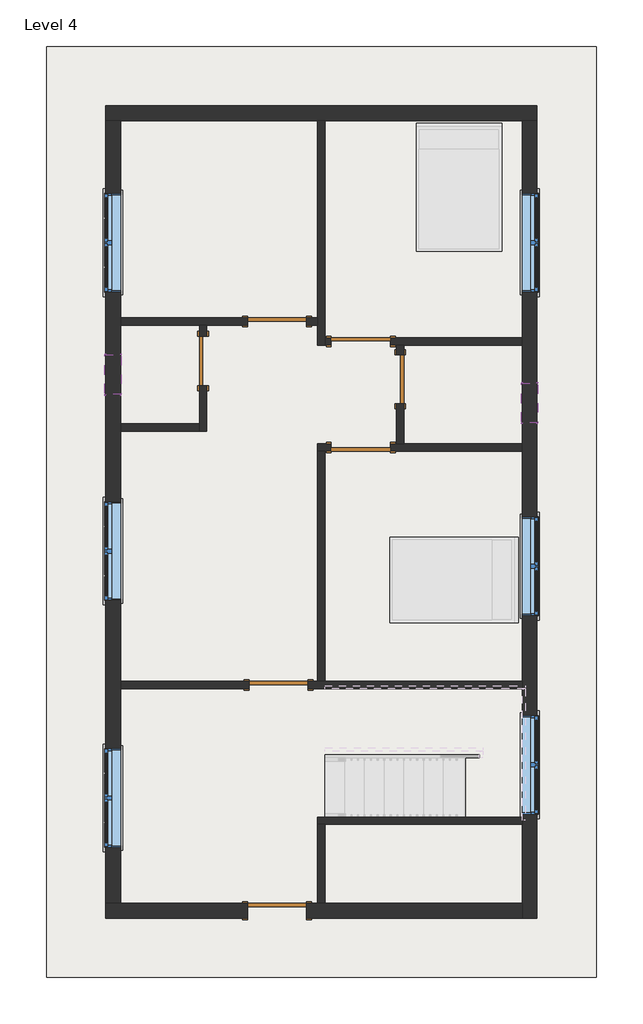
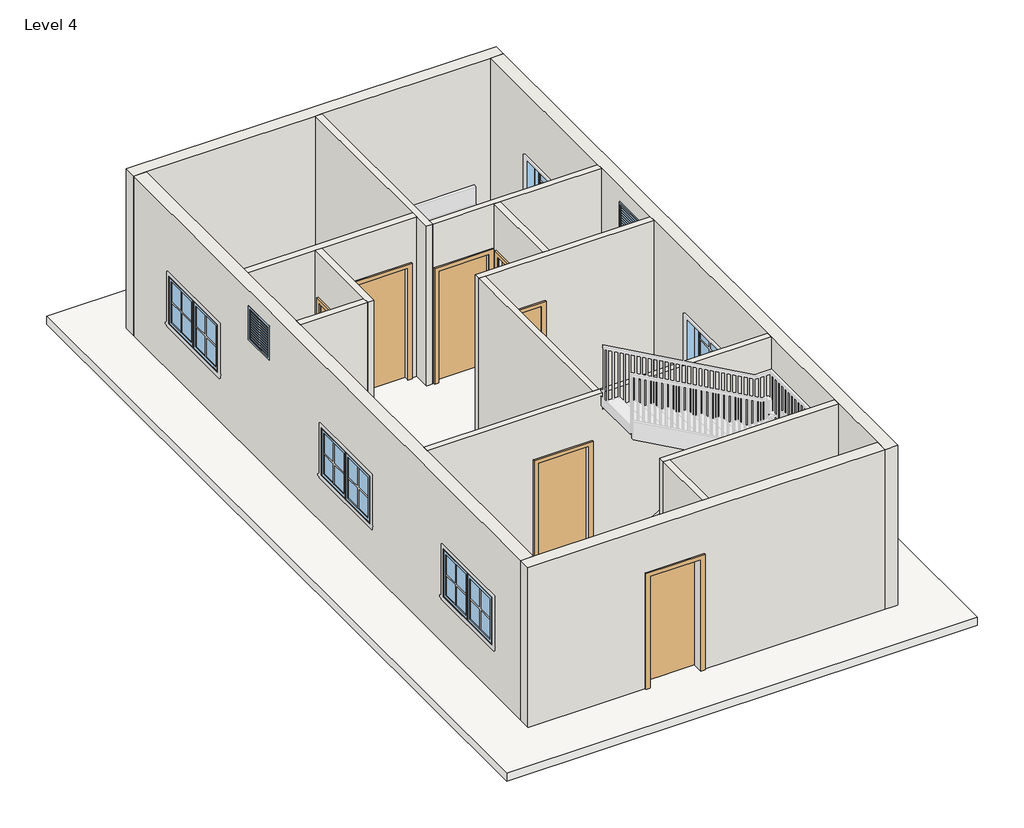
# One storey, part 1 of 3: 15 walls, 8 windows, 7 doors, 1 roof.
"""IFC4 building model written with IfcOpenShell, lengths in millimetres."""

from ifc_helpers import new_model, si_unit, frame, origin, place, context, project, spatial, polyline, outline, extrude, faceted_brep, transform, mapped, element, save
from components import door_78caadf7, door_214872d5, single_flush_door_3_e5f9f3c4, single_flush_door_3_305aa2a5, single_flush_door_3_0ca8825f, window_casement_double_win_5_c1d95f0f, window_f2d8fef0

model = new_model("IFC4")

# Units and contexts
model_context = context("Model", 3, world=origin())
ifc_project = project(units=[si_unit("LENGTHUNIT", "METRE", prefix="MILLI")], contexts=[model_context])

# Site, building, storey
site = spatial("IfcSite", under=ifc_project)
building = spatial("IfcBuilding", under=site)
storey = spatial("IfcBuildingStorey", under=building, Name="Level 4", Elevation=9448.8)

# Doors
placement = place(None, origin())
door_shape = door_78caadf7(model_context)
element("IfcDoor", 1, ObjectType="Single-Flush : 2'6\"", at=placement, inside=storey, context=model_context, shape_type="MappedRepresentation", body=[
    mapped(door_shape, transform((-35.92188, 1946.24131, 9448.8), x_axis=(0.0, 1.0, 0.0), y_axis=(-1.0, 0.0, 0.0), z_axis=(0.0, 0.0, 1.0))),
])
door_2_shape = door_214872d5(model_context)
element("IfcDoor", 2, ObjectType="Single-Flush : 2'6\"", at=placement, inside=storey, context=model_context, shape_type="MappedRepresentation", body=[
    mapped(door_2_shape, transform((-3083.92188, 2225.64131, 9448.8), x_axis=(0.0, 1.0, 0.0), y_axis=(-1.0, 0.0, 0.0), z_axis=(0.0, 0.0, 1.0))),
])
single_flush_door_3_shape = single_flush_door_3_e5f9f3c4(model_context)
element("IfcDoor", 3, ObjectType="Single-Flush : DOOR 3'", at=placement, inside=storey, context=model_context, shape_type="MappedRepresentation", body=[
    mapped(single_flush_door_3_shape, transform((-1940.92188, 2835.24131, 9448.8), x_axis=(1.0, 0.0, 0.0), y_axis=(0.0, 1.0, 0.0), z_axis=(0.0, 0.0, 1.0))),
])
element("IfcDoor", 4, ObjectType="Single-Flush : DOOR 3'", at=placement, inside=storey, context=model_context, shape_type="MappedRepresentation", body=[
    mapped(single_flush_door_3_shape, transform((-645.52188, 892.14131, 9448.8), x_axis=(-1.0, 0.0, 0.0), y_axis=(0.0, -1.0, 0.0), z_axis=(0.0, 0.0, 1.0))),
])
element("IfcDoor", 5, ObjectType="Single-Flush : DOOR 3'", at=placement, inside=storey, context=model_context, shape_type="MappedRepresentation", body=[
    mapped(single_flush_door_3_shape, transform((-1915.52188, -2778.15869, 9448.8), x_axis=(1.0, 0.0, 0.0), y_axis=(0.0, 1.0, 0.0), z_axis=(0.0, 0.0, 1.0))),
])
single_flush_door_3_2_shape = single_flush_door_3_305aa2a5(model_context)
element("IfcDoor", 6, ObjectType="Single-Flush : DOOR 3'", at=placement, inside=storey, context=model_context, shape_type="MappedRepresentation", body=[
    mapped(single_flush_door_3_2_shape, transform((-645.52188, 2530.44131, 9448.8), x_axis=(-1.0, 0.0, 0.0), y_axis=(0.0, -1.0, 0.0), z_axis=(0.0, 0.0, 1.0))),
])
single_flush_door_3_3_shape = single_flush_door_3_0ca8825f(model_context)
element("IfcDoor", 7, ObjectType="Single-Flush : DOOR 3'", at=placement, inside=storey, context=model_context, shape_type="MappedRepresentation", body=[
    mapped(single_flush_door_3_3_shape, transform((-1940.92188, -6264.30869, 9448.8), x_axis=(1.0, 0.0, 0.0), y_axis=(0.0, 1.0, 0.0), z_axis=(0.0, 0.0, 1.0))),
])

# Roof
element("IfcRoof", 8, ObjectType="ROOF 6\"", at=placement, inside=storey, context=model_context, shape_type="SweptSolid", body=[
    extrude(outline(polyline([(-5503.27188, 7083.39131), (2993.02812, 7083.39131), (2993.02812, -7293.00869), (-5503.27188, -7293.00869), (-5503.27188, 7083.39131)])), frame((0.0, 0.0, 9296.4), z_axis=(0.0, 0.0, 1.0), x_axis=(1.0, 0.0, 0.0)), (0.0, 0.0, 1.0), 152.4),
])

# Walls
element("IfcWall", 9, ObjectType="WALL 4.5'", at=placement, inside=storey, context=model_context, shape_type="Brep", body=[
    faceted_brep([(-1312.27188, 5940.39131, 9448.8), (-1312.27188, 2892.39131, 9448.8), (-1312.27188, 2778.09131, 9448.8), (-1312.27188, 2473.29131, 9448.8), (-1312.27188, 2473.29131, 12496.8), (-1312.27188, 2778.09131, 12496.8), (-1312.27188, 2892.39131, 12496.8), (-1312.27188, 5940.39131, 12496.8), (-1197.97188, 5940.39131, 9448.8), (-1197.97188, 5940.39131, 12496.8), (-1197.97188, 2587.59131, 12496.8), (-1197.97188, 2473.29131, 12496.8), (-1197.97188, 2473.29131, 9448.8), (-1197.97188, 2587.59131, 9448.8)], [[[0, 1, 2, 3, 4, 5, 6, 7]], [[8, 9, 10, 11, 12, 13]], [[3, 2, 1, 0, 8, 13, 12]], [[0, 7, 9, 8]], [[4, 3, 12, 11]], [[7, 6, 5, 4, 11, 10, 9]]]),
])
element("IfcWall", 10, ObjectType="WALL 4.5'", at=placement, inside=storey, context=model_context, shape_type="Brep", body=[
    faceted_brep([(-1197.97188, 2473.29131, 9448.8), (-1102.72188, 2473.29131, 9448.8), (-1102.72188, 2473.29131, 11582.4), (-188.32188, 2473.29131, 11582.4), (-188.32188, 2473.29131, 9448.8), (-93.07188, 2473.29131, 9448.8), (21.22812, 2473.29131, 9448.8), (1850.02812, 2473.29131, 9448.8), (1850.02812, 2473.29131, 12496.8), (21.22812, 2473.29131, 12496.8), (-93.07188, 2473.29131, 12496.8), (-1197.97188, 2473.29131, 12496.8), (-1102.72188, 2587.59131, 11582.4), (-1102.72188, 2587.59131, 9448.8), (-1197.97188, 2587.59131, 9448.8), (-1197.97188, 2587.59131, 12496.8), (1850.02812, 2587.59131, 12496.8), (1850.02812, 2587.59131, 9448.8), (-188.32188, 2587.59131, 9448.8), (-188.32188, 2587.59131, 11582.4)], [[[0, 1, 2, 3, 4, 5, 6, 7, 8, 9, 10, 11]], [[12, 13, 14, 15, 16, 17, 18, 19]], [[18, 17, 7, 6, 5, 4]], [[14, 13, 1, 0]], [[0, 11, 15, 14]], [[8, 7, 17, 16]], [[2, 1, 13, 12]], [[3, 2, 12, 19]], [[4, 3, 19, 18]], [[11, 10, 9, 8, 16, 15]]]),
])
element("IfcWall", 11, ObjectType="WALL 4.5'", at=placement, inside=storey, context=model_context, shape_type="Brep", body=[
    faceted_brep([(-1312.27188, 2892.39131, 9448.8), (-1483.72188, 2892.39131, 9448.8), (-1483.72188, 2892.39131, 11582.4), (-2398.12188, 2892.39131, 11582.4), (-2398.12188, 2892.39131, 9448.8), (-4360.27188, 2892.39131, 9448.8), (-4360.27188, 2892.39131, 12496.8), (-1312.27188, 2892.39131, 12496.8), (-1483.72188, 2778.09131, 11582.4), (-1483.72188, 2778.09131, 9448.8), (-1312.27188, 2778.09131, 9448.8), (-1312.27188, 2778.09131, 12496.8), (-3026.77188, 2778.09131, 12496.8), (-3141.07188, 2778.09131, 12496.8), (-4360.27188, 2778.09131, 12496.8), (-4360.27188, 2778.09131, 9448.8), (-3141.07188, 2778.09131, 9448.8), (-3026.77188, 2778.09131, 9448.8), (-2398.12188, 2778.09131, 9448.8), (-2398.12188, 2778.09131, 11582.4)], [[[0, 1, 2, 3, 4, 5, 6, 7]], [[8, 9, 10, 11, 12, 13, 14, 15, 16, 17, 18, 19]], [[10, 9, 1, 0]], [[18, 17, 16, 15, 5, 4]], [[6, 5, 15, 14]], [[0, 7, 11, 10]], [[2, 1, 9, 8]], [[3, 2, 8, 19]], [[4, 3, 19, 18]], [[7, 6, 14, 13, 12, 11]]]),
])
element("IfcWall", 12, ObjectType="WALL 4.5'", at=placement, inside=storey, context=model_context, shape_type="Brep", body=[
    faceted_brep([(-3141.07188, 2778.09131, 9448.8), (-3141.07188, 2606.64131, 9448.8), (-3141.07188, 2606.64131, 11582.4), (-3141.07188, 1844.64131, 11582.4), (-3141.07188, 1844.64131, 9448.8), (-3141.07188, 1254.09131, 9448.8), (-3141.07188, 1139.79131, 9448.8), (-3141.07188, 1139.79131, 12496.8), (-3141.07188, 1254.09131, 12496.8), (-3141.07188, 2778.09131, 12496.8), (-3026.77188, 2606.64131, 11582.4), (-3026.77188, 2606.64131, 9448.8), (-3026.77188, 2778.09131, 9448.8), (-3026.77188, 2778.09131, 12496.8), (-3026.77188, 1139.79131, 12496.8), (-3026.77188, 1139.79131, 9448.8), (-3026.77188, 1844.64131, 9448.8), (-3026.77188, 1844.64131, 11582.4)], [[[0, 1, 2, 3, 4, 5, 6, 7, 8, 9]], [[10, 11, 12, 13, 14, 15, 16, 17]], [[16, 15, 6, 5, 4]], [[12, 11, 1, 0]], [[0, 9, 13, 12]], [[7, 6, 15, 14]], [[2, 1, 11, 10]], [[3, 2, 10, 17]], [[4, 3, 17, 16]], [[9, 8, 7, 14, 13]]]),
])
element("IfcWall", 13, ObjectType="WALL 4.5'", at=placement, inside=storey, context=model_context, shape_type="SweptSolid", body=[
    extrude(outline(polyline([(-4360.27188, 1254.09131), (-3141.07188, 1254.09131), (-3141.07188, 1139.79131), (-4360.27188, 1139.79131), (-4360.27188, 1254.09131)])), frame((0.0, 0.0, 9448.8), z_axis=(0.0, 0.0, 1.0), x_axis=(1.0, 0.0, 0.0)), (0.0, 0.0, 1.0), 3048.0),
])
element("IfcWall", 14, ObjectType="WALL 4.5'", at=placement, inside=storey, context=model_context, shape_type="SweptSolid", body=[
    extrude(outline(polyline([(2473.29131, 9448.8), (2327.24131, 9448.8), (2327.24131, 11582.4), (1565.24131, 11582.4), (1565.24131, 9448.8), (949.29131, 9448.8), (949.29131, 12496.8), (2473.29131, 12496.8), (2473.29131, 9448.8)])), frame((-93.07188, 0.0, 0.0), z_axis=(1.0, 0.0, 0.0), x_axis=(0.0, 1.0, 0.0)), (0.0, 0.0, 1.0), 114.3),
])
element("IfcWall", 15, ObjectType="WALL 4.5'", at=placement, inside=storey, context=model_context, shape_type="Brep", body=[
    faceted_brep([(-1102.72188, 949.29131, 11582.4), (-1102.72188, 949.29131, 9448.8), (-1312.27188, 949.29131, 9448.8), (-1312.27188, 949.29131, 12496.8), (-93.07188, 949.29131, 12496.8), (21.22812, 949.29131, 12496.8), (1850.02812, 949.29131, 12496.8), (1850.02812, 949.29131, 9448.8), (21.22812, 949.29131, 9448.8), (-93.07188, 949.29131, 9448.8), (-188.32188, 949.29131, 9448.8), (-188.32188, 949.29131, 11582.4), (-1312.27188, 834.99131, 9448.8), (-1197.97188, 834.99131, 9448.8), (-1102.72188, 834.99131, 9448.8), (-1102.72188, 834.99131, 11582.4), (-188.32188, 834.99131, 11582.4), (-188.32188, 834.99131, 9448.8), (1850.02812, 834.99131, 9448.8), (1850.02812, 834.99131, 12496.8), (-1197.97188, 834.99131, 12496.8), (-1312.27188, 834.99131, 12496.8)], [[[0, 1, 2, 3, 4, 5, 6, 7, 8, 9, 10, 11]], [[12, 13, 14, 15, 16, 17, 18, 19, 20, 21]], [[2, 1, 14, 13, 12]], [[10, 9, 8, 7, 18, 17]], [[7, 6, 19, 18]], [[3, 2, 12, 21]], [[15, 14, 1, 0]], [[16, 15, 0, 11]], [[17, 16, 11, 10]], [[6, 5, 4, 3, 21, 20, 19]]]),
])
element("IfcWall", 16, ObjectType="WALL 4.5'", at=placement, inside=storey, context=model_context, shape_type="SweptSolid", body=[
    extrude(outline(polyline([(-1312.27188, -2721.00869), (-1312.27188, 834.99131), (-1197.97188, 834.99131), (-1197.97188, -2721.00869), (-1312.27188, -2721.00869)])), frame((0.0, 0.0, 9448.8), z_axis=(0.0, 0.0, 1.0), x_axis=(1.0, 0.0, 0.0)), (0.0, 0.0, 1.0), 3048.0),
])
element("IfcWall", 17, ObjectType="WALL 4.5'", at=placement, inside=storey, context=model_context, shape_type="Brep", body=[
    faceted_brep([(1850.02812, -2721.00869, 9448.8), (-1197.97188, -2721.00869, 9448.8), (-1312.27188, -2721.00869, 9448.8), (-1458.32188, -2721.00869, 9448.8), (-1458.32188, -2721.00869, 11582.4), (-2372.72188, -2721.00869, 11582.4), (-2372.72188, -2721.00869, 9448.8), (-4360.27188, -2721.00869, 9448.8), (-4360.27188, -2721.00869, 12496.8), (-1312.27188, -2721.00869, 12496.8), (-1197.97188, -2721.00869, 12496.8), (1850.02812, -2721.00869, 12496.8), (-1458.32188, -2835.30869, 11582.4), (-1458.32188, -2835.30869, 9448.8), (1850.02812, -2835.30869, 9448.8), (1850.02812, -2835.30869, 12496.8), (-4360.27188, -2835.30869, 12496.8), (-4360.27188, -2835.30869, 9448.8), (-2372.72188, -2835.30869, 9448.8), (-2372.72188, -2835.30869, 11582.4)], [[[0, 1, 2, 3, 4, 5, 6, 7, 8, 9, 10, 11]], [[12, 13, 14, 15, 16, 17, 18, 19]], [[18, 17, 7, 6]], [[14, 13, 3, 2, 1, 0]], [[0, 11, 15, 14]], [[8, 7, 17, 16]], [[4, 3, 13, 12]], [[5, 4, 12, 19]], [[6, 5, 19, 18]], [[11, 10, 9, 8, 16, 15]]]),
])
element("IfcWall", 18, ObjectType="WALL 4.5'", at=placement, inside=storey, context=model_context, shape_type="Brep", body=[
    faceted_brep([(1850.02812, -4816.50869, 9448.8), (-1312.27188, -4816.50869, 9448.8), (-1312.27188, -4816.50869, 12496.8), (1850.02812, -4816.50869, 12496.8), (1850.02812, -4930.80869, 9448.8), (1850.02812, -4930.80869, 12496.8), (-1197.97188, -4930.80869, 12496.8), (-1312.27188, -4930.80869, 12496.8), (-1312.27188, -4930.80869, 9448.8), (-1197.97188, -4930.80869, 9448.8)], [[[0, 1, 2, 3]], [[4, 5, 6, 7, 8, 9]], [[1, 0, 4, 9, 8]], [[0, 3, 5, 4]], [[2, 1, 8, 7]], [[3, 2, 7, 6, 5]]]),
])
element("IfcWall", 19, ObjectType="WALL 4.5'", at=placement, inside=storey, context=model_context, shape_type="SweptSolid", body=[
    extrude(outline(polyline([(-1312.27188, -6150.00869), (-1312.27188, -4930.80869), (-1197.97188, -4930.80869), (-1197.97188, -6150.00869), (-1312.27188, -6150.00869)])), frame((0.0, 0.0, 9448.8), z_axis=(0.0, 0.0, 1.0), x_axis=(1.0, 0.0, 0.0)), (0.0, 0.0, 1.0), 3048.0),
])
element("IfcWall", 20, ObjectType="WALL 9\"", at=placement, inside=storey, context=model_context, shape_type="Brep", body=[
    faceted_brep([(-4588.87188, 5940.39131, 9448.8), (-4360.27188, 5940.39131, 9448.8), (-1312.27188, 5940.39131, 9448.8), (-1197.97188, 5940.39131, 9448.8), (1850.02812, 5940.39131, 9448.8), (2078.62812, 5940.39131, 9448.8), (2078.62812, 5940.39131, 12496.8), (1850.02812, 5940.39131, 12496.8), (-1197.97188, 5940.39131, 12496.8), (-1312.27188, 5940.39131, 12496.8), (-4360.27188, 5940.39131, 12496.8), (-4588.87188, 5940.39131, 12496.8), (-4588.87188, 6168.99131, 9448.8), (-4588.87188, 6168.99131, 12496.8), (2078.62812, 6168.99131, 12496.8), (2078.62812, 6168.99131, 9448.8)], [[[0, 1, 2, 3, 4, 5, 6, 7, 8, 9, 10, 11]], [[12, 13, 14, 15]], [[5, 4, 3, 2, 1, 0, 12, 15]], [[6, 5, 15, 14]], [[0, 11, 13, 12]], [[11, 10, 9, 8, 7, 6, 14, 13]]]),
])
element("IfcWall", 21, ObjectType="WALL 9\"", at=placement, inside=storey, context=model_context, shape_type="Brep", body=[
    faceted_brep([(1850.02812, 5940.39131, 9448.8), (1850.02812, 2587.59131, 9448.8), (1850.02812, 2473.29131, 9448.8), (1850.02812, 949.29131, 9448.8), (1850.02812, 834.99131, 9448.8), (1850.02812, -2721.00869, 9448.8), (1850.02812, -2835.30869, 9448.8), (1850.02812, -4816.50869, 9448.8), (1850.02812, -4930.80869, 9448.8), (1850.02812, -6150.00869, 9448.8), (1850.02812, -6378.60869, 9448.8), (1850.02812, -6378.60869, 12496.8), (1850.02812, -6150.00869, 12496.8), (1850.02812, -4930.80869, 12496.8), (1850.02812, -4816.50869, 12496.8), (1850.02812, -2835.30869, 12496.8), (1850.02812, -2721.00869, 12496.8), (1850.02812, 834.99131, 12496.8), (1850.02812, 949.29131, 12496.8), (1850.02812, 2473.29131, 12496.8), (1850.02812, 2587.59131, 12496.8), (1850.02812, 5940.39131, 12496.8), (1850.02812, -4772.05869, 11277.6), (1850.02812, -4772.05869, 10363.2), (1850.02812, -3248.05869, 10363.2), (1850.02812, -3248.05869, 11277.6), (1850.02812, 3292.44131, 11277.6), (1850.02812, 3292.44131, 10363.2), (1850.02812, 4816.44131, 10363.2), (1850.02812, 4816.44131, 11277.6), (1850.02812, -1705.00869, 11277.6), (1850.02812, -1705.00869, 10363.2), (1850.02812, -181.00869, 10363.2), (1850.02812, -181.00869, 11277.6), (1850.02812, 1273.14131, 12192.0), (1850.02812, 1273.14131, 11582.4), (1850.02812, 1882.74131, 11582.4), (1850.02812, 1882.74131, 12192.0), (2078.62812, 5940.39131, 9448.8), (2078.62812, 5940.39131, 12496.8), (2078.62812, -6378.60869, 12496.8), (2078.62812, -6378.60869, 9448.8), (2078.62812, -4772.05869, 11277.6), (2078.62812, -3248.05869, 11277.6), (2078.62812, -3248.05869, 10363.2), (2078.62812, -4772.05869, 10363.2), (2078.62812, 3292.44131, 11277.6), (2078.62812, 4816.44131, 11277.6), (2078.62812, 4816.44131, 10363.2), (2078.62812, 3292.44131, 10363.2), (2078.62812, -1705.00869, 11277.6), (2078.62812, -181.00869, 11277.6), (2078.62812, -181.00869, 10363.2), (2078.62812, -1705.00869, 10363.2), (2078.62812, 1273.14131, 12192.0), (2078.62812, 1882.74131, 12192.0), (2078.62812, 1882.74131, 11582.4), (2078.62812, 1273.14131, 11582.4)], [[[0, 1, 2, 3, 4, 5, 6, 7, 8, 9, 10, 11, 12, 13, 14, 15, 16, 17, 18, 19, 20, 21], [22, 23, 24, 25], [26, 27, 28, 29], [30, 31, 32, 33], [34, 35, 36, 37]], [[38, 39, 40, 41], [42, 43, 44, 45], [46, 47, 48, 49], [50, 51, 52, 53], [54, 55, 56, 57]], [[10, 9, 8, 7, 6, 5, 4, 3, 2, 1, 0, 38, 41]], [[0, 21, 39, 38]], [[11, 10, 41, 40]], [[23, 22, 42, 45]], [[24, 23, 45, 44]], [[25, 24, 44, 43]], [[22, 25, 43, 42]], [[27, 26, 46, 49]], [[28, 27, 49, 48]], [[29, 28, 48, 47]], [[26, 29, 47, 46]], [[31, 30, 50, 53]], [[32, 31, 53, 52]], [[33, 32, 52, 51]], [[30, 33, 51, 50]], [[35, 34, 54, 57]], [[36, 35, 57, 56]], [[37, 36, 56, 55]], [[34, 37, 55, 54]], [[21, 20, 19, 18, 17, 16, 15, 14, 13, 12, 11, 40, 39]]]),
])
element("IfcWall", 22, ObjectType="WALL 9\"", at=placement, inside=storey, context=model_context, shape_type="Brep", body=[
    faceted_brep([(1850.02812, -6150.00869, 9448.8), (-1197.97188, -6150.00869, 9448.8), (-1312.27188, -6150.00869, 9448.8), (-1483.72188, -6150.00869, 9448.8), (-1483.72188, -6150.00869, 11582.4), (-2398.12188, -6150.00869, 11582.4), (-2398.12188, -6150.00869, 9448.8), (-4360.27188, -6150.00869, 9448.8), (-4588.87188, -6150.00869, 9448.8), (-4588.87188, -6150.00869, 12496.8), (-4360.27188, -6150.00869, 12496.8), (-1312.27188, -6150.00869, 12496.8), (-1197.97188, -6150.00869, 12496.8), (1850.02812, -6150.00869, 12496.8), (-1483.72188, -6378.60869, 11582.4), (-1483.72188, -6378.60869, 9448.8), (1850.02812, -6378.60869, 9448.8), (1850.02812, -6378.60869, 12496.8), (-4588.87188, -6378.60869, 12496.8), (-4588.87188, -6378.60869, 9448.8), (-2398.12188, -6378.60869, 9448.8), (-2398.12188, -6378.60869, 11582.4)], [[[0, 1, 2, 3, 4, 5, 6, 7, 8, 9, 10, 11, 12, 13]], [[14, 15, 16, 17, 18, 19, 20, 21]], [[20, 19, 8, 7, 6]], [[16, 15, 3, 2, 1, 0]], [[0, 13, 17, 16]], [[9, 8, 19, 18]], [[4, 3, 15, 14]], [[5, 4, 14, 21]], [[6, 5, 21, 20]], [[13, 12, 11, 10, 9, 18, 17]]]),
])
element("IfcWall", 23, ObjectType="WALL 9\"", at=placement, inside=storey, context=model_context, shape_type="Brep", body=[
    faceted_brep([(-4360.27188, -6150.00869, 9448.8), (-4360.27188, -2835.30869, 9448.8), (-4360.27188, -2721.00869, 9448.8), (-4360.27188, 1139.79131, 9448.8), (-4360.27188, 1254.09131, 9448.8), (-4360.27188, 2778.09131, 9448.8), (-4360.27188, 2892.39131, 9448.8), (-4360.27188, 5940.39131, 9448.8), (-4360.27188, 5940.39131, 12496.8), (-4360.27188, 2892.39131, 12496.8), (-4360.27188, 2778.09131, 12496.8), (-4360.27188, 1254.09131, 12496.8), (-4360.27188, 1139.79131, 12496.8), (-4360.27188, -2721.00869, 12496.8), (-4360.27188, -2835.30869, 12496.8), (-4360.27188, -6150.00869, 12496.8), (-4360.27188, 4816.44131, 11277.6), (-4360.27188, 4816.44131, 10363.2), (-4360.27188, 3292.44131, 10363.2), (-4360.27188, 3292.44131, 11277.6), (-4360.27188, 53.94131, 11277.6), (-4360.27188, 53.94131, 10363.2), (-4360.27188, -1470.05869, 10363.2), (-4360.27188, -1470.05869, 11277.6), (-4360.27188, -3759.23369, 11277.6), (-4360.27188, -3759.23369, 10363.2), (-4360.27188, -5283.23369, 10363.2), (-4360.27188, -5283.23369, 11277.6), (-4360.27188, 1711.29131, 12192.0), (-4360.27188, 2320.89131, 12192.0), (-4360.27188, 2320.89131, 11582.4), (-4360.27188, 1711.29131, 11582.4), (-4588.87188, -6150.00869, 9448.8), (-4588.87188, -6150.00869, 12496.8), (-4588.87188, 5940.39131, 12496.8), (-4588.87188, 5940.39131, 9448.8), (-4588.87188, 4816.44131, 11277.6), (-4588.87188, 3292.44131, 11277.6), (-4588.87188, 3292.44131, 10363.2), (-4588.87188, 4816.44131, 10363.2), (-4588.87188, 53.94131, 11277.6), (-4588.87188, -1470.05869, 11277.6), (-4588.87188, -1470.05869, 10363.2), (-4588.87188, 53.94131, 10363.2), (-4588.87188, -3759.23369, 11277.6), (-4588.87188, -5283.23369, 11277.6), (-4588.87188, -5283.23369, 10363.2), (-4588.87188, -3759.23369, 10363.2), (-4588.87188, 1711.29131, 12192.0), (-4588.87188, 1711.29131, 11582.4), (-4588.87188, 2320.89131, 11582.4), (-4588.87188, 2320.89131, 12192.0)], [[[0, 1, 2, 3, 4, 5, 6, 7, 8, 9, 10, 11, 12, 13, 14, 15], [16, 17, 18, 19], [20, 21, 22, 23], [24, 25, 26, 27], [28, 29, 30, 31]], [[32, 33, 34, 35], [36, 37, 38, 39], [40, 41, 42, 43], [44, 45, 46, 47], [48, 49, 50, 51]], [[7, 6, 5, 4, 3, 2, 1, 0, 32, 35]], [[8, 7, 35, 34]], [[0, 15, 33, 32]], [[17, 16, 36, 39]], [[18, 17, 39, 38]], [[19, 18, 38, 37]], [[16, 19, 37, 36]], [[21, 20, 40, 43]], [[22, 21, 43, 42]], [[23, 22, 42, 41]], [[20, 23, 41, 40]], [[25, 24, 44, 47]], [[26, 25, 47, 46]], [[27, 26, 46, 45]], [[24, 27, 45, 44]], [[49, 48, 28, 31]], [[50, 49, 31, 30]], [[51, 50, 30, 29]], [[48, 51, 29, 28]], [[15, 14, 13, 12, 11, 10, 9, 8, 34, 33]]]),
])

# Windows
window_casement_double_win_5_shape = window_casement_double_win_5_c1d95f0f(model_context)
element("IfcWindow", 24, ObjectType="Window-Casement-Double : WIN 5'", at=placement, inside=storey, context=model_context, shape_type="MappedRepresentation", body=[
    mapped(window_casement_double_win_5_shape, transform((-4474.57188, 4054.44131, 9448.8), x_axis=(0.0, 1.0, 0.0), y_axis=(-1.0, 0.0, 0.0), z_axis=(0.0, 0.0, 1.0))),
])
element("IfcWindow", 25, ObjectType="Window-Casement-Double : WIN 5'", at=placement, inside=storey, context=model_context, shape_type="MappedRepresentation", body=[
    mapped(window_casement_double_win_5_shape, transform((-4474.57188, -708.05869, 9448.8), x_axis=(0.0, 1.0, 0.0), y_axis=(-1.0, 0.0, 0.0), z_axis=(0.0, 0.0, 1.0))),
])
element("IfcWindow", 26, ObjectType="Window-Casement-Double : WIN 5'", at=placement, inside=storey, context=model_context, shape_type="MappedRepresentation", body=[
    mapped(window_casement_double_win_5_shape, transform((-4474.57188, -4521.23369, 9448.8), x_axis=(0.0, 1.0, 0.0), y_axis=(-1.0, 0.0, 0.0), z_axis=(0.0, 0.0, 1.0))),
])
element("IfcWindow", 27, ObjectType="Window-Casement-Double : WIN 5'", at=placement, inside=storey, context=model_context, shape_type="MappedRepresentation", body=[
    mapped(window_casement_double_win_5_shape, transform((1964.32812, -4010.05869, 9448.8), x_axis=(0.0, -1.0, 0.0), y_axis=(1.0, 0.0, 0.0), z_axis=(0.0, 0.0, 1.0))),
])
element("IfcWindow", 28, ObjectType="Window-Casement-Double : WIN 5'", at=placement, inside=storey, context=model_context, shape_type="MappedRepresentation", body=[
    mapped(window_casement_double_win_5_shape, transform((1964.32812, 4054.44131, 9448.8), x_axis=(0.0, -1.0, 0.0), y_axis=(1.0, 0.0, 0.0), z_axis=(0.0, 0.0, 1.0))),
])
element("IfcWindow", 29, ObjectType="Window-Casement-Double : WIN 5'", at=placement, inside=storey, context=model_context, shape_type="MappedRepresentation", body=[
    mapped(window_casement_double_win_5_shape, transform((1964.32812, -943.00869, 9448.8), x_axis=(0.0, -1.0, 0.0), y_axis=(1.0, 0.0, 0.0), z_axis=(0.0, 0.0, 1.0))),
])
window_shape = window_f2d8fef0(model_context)
element("IfcWindow", 30, ObjectType="Window-Louvers : 24\" x 24\"", at=placement, inside=storey, context=model_context, shape_type="MappedRepresentation", body=[
    mapped(window_shape, transform((1957.97812, 1577.94131, 10668.0), x_axis=(0.0, 1.0, 0.0), y_axis=(-1.0, 0.0, 0.0), z_axis=(0.0, 0.0, 1.0))),
])
element("IfcWindow", 31, ObjectType="Window-Louvers : 24\" x 24\"", at=placement, inside=storey, context=model_context, shape_type="MappedRepresentation", body=[
    mapped(window_shape, transform((-4480.92188, 2016.09131, 10668.0), x_axis=(0.0, 1.0, 0.0), y_axis=(-1.0, 0.0, 0.0), z_axis=(0.0, 0.0, 1.0))),
])

save(model, "model.ifc")

# Revit data of these elements
# Type "Single-Flush : 2'6\""
#   Type Mark = "9"
#   Construction Type Id = "MDOOR"
#   Assembly Code = "C1020"
#   Analytic Construction = "Metal"
#   Thickness = 0' - 2"
#   Heat Transfer Coefficient (U) = 0.651978 BTU/(h·ft²·°F)
#   Height = 7' - 0"
#   Trim Projection Ext = 0' - 1"
#   Trim Projection Int = 0' - 1"
#   Trim Width = 0' - 3"
#   Width = 2' - 6"
#   Define Thermal Properties by = 1
#   Door Material = Door - Panel
#   Frame Material = Door - Frame
#   Visual Light Transmittance = 0
#   Solar Heat Gain Coefficient = 0
#   Function = (empty or 0)
#   Wall Closure = (empty or 0)
# Type "Single-Flush : DOOR 3'"
#   Type Mark = "8"
#   Construction Type Id = "MDOOR"
#   Assembly Code = "C1020"
#   Analytic Construction = "Metal"
#   Thickness = 0' - 2"
#   Heat Transfer Coefficient (U) = 0.651978 BTU/(h·ft²·°F)
#   Height = 7' - 0"
#   Trim Projection Ext = 0' - 1"
#   Trim Projection Int = 0' - 1"
#   Trim Width = 0' - 3"
#   Width = 3' - 0"
#   Define Thermal Properties by = 1
#   Door Material = Door - Panel
#   Frame Material = Door - Frame
#   Visual Light Transmittance = 0
#   Solar Heat Gain Coefficient = 0
#   Function = (empty or 0)
#   Wall Closure = (empty or 0)
# Type "ROOF 6\""
#   Assembly Code = "B1020"
#   Layers, outside or top first: 0' - 6" no material (function 1)
# Type "WALL 4.5'"
#   Assembly Code = "B2010"
#   Layers, outside or top first: 0' - 4 1/2" no material (function 1)
# Type "WALL 9\""
#   Assembly Code = "B2010"
#   Layers, outside or top first: 0' - 9" no material (function 1)
# Type "Window-Casement-Double : WIN 5'"
#   Type Mark = "18"
#   Fire Rating = "0.5h"
#   Assembly Code = "B2020100"
#   Analytic Construction = "Double glazing - domestic"
#   Frame Extension [instance default] = 0' - 0 1/4"
#   Window Inset [instance default] = 0' - 0"
#   Wall Thickness [instance default] = 0' - 6"
#   Interior Wall Closure [instance default] = 0' - 2 1/4"
#   Half Width = 2' - 6"
#   Visual Light Transmittance = 0.81
#   Thermal Resistance (R) = 1.8146 (h·ft²·°F)/BTU
#   Solar Heat Gain Coefficient = 0.76
#   Rough Width = 5' - 0 1/2"
#   Rough Height = 3' - 0 1/2"
#   Height = 3' - 0"
#   Heat Transfer Coefficient (U) = 0.5511 BTU/(h·ft²·°F)
#   Exterior Wall Closure [instance default] = 0' - 1 1/4"
#   Extension Jamb [instance default] = 0' - 2 1/4"
#   Default Sill Height = 3' - 0"
#   Width = 5' - 0"
#   Muntin Visibility = yes
#   Interior Trim Visibility [instance default] = yes
#   Exterior Trim Visibility [instance default] = yes
#   Extension Jamb Visibility [instance default] = yes
#   Interior Trim Material = Wood - Stained
#   Muntin Pattern = Muntin Pattern_2x2 : Muntin Pattern_2x2
#   Interior Trim = Trim-Window-Interior-Flat : Picture Frame
#   Interior Frame Material = Wood - Stained
#   Glass Panel Material = Glass
#   Exterior Trim Material = Clad - White
#   Exterior Trim = Trim-Window-Exterior-Flat : with Sill
#   Exterior Frame Material = Clad - White
#   Wall Closure = (empty or 0)
# Type "Window-Louvers : 24\" x 24\""
#   Type Mark = "19"
#   Construction Type Id = "GSP4R"
#   Assembly Code = "B20"
#   Analytic Construction = "1/8 in Pilkington single glazing"
#   Visual Light Transmittance = 0.9
#   Thermal Resistance (R) = 1.53941 (h·ft²·°F)/BTU
#   Solar Heat Gain Coefficient = 0.78
#   Max Height = 1' - 11.74264"
#   Height = 2' - 0"
#   Heat Transfer Coefficient (U) = 0.6496 BTU/(h·ft²·°F)
#   Blade Width [instance default] = 1' - 10 1/2"
#   Blade Vertical Thickness = 0' - 0.35355"
#   Blade Thickness = 0' - 0 1/4"
#   Blade Spacing = 0' - 1 1/2"
#   Blade Height = 0' - 1.85355"
#   Blade Depth = 0' - 3"
#   Blade Angle = 45.00°
#   Default Sill Height = 3' - 0"
#   Trim Projection_Exterior = 0' - 0 1/2"
#   Trim Projection_Interior = 0' - 0 1/2"
#   Trim Width_Exterior = 0' - 1 1/2"
#   Trim Width_Interior = 0' - 1 1/2"
#   Width = 2' - 0"
#   Max Blade Count = 12
#   Define Thermal Properties by = 1
#   Blade Count = 12
#   Frame Material = Birch
#   Louver Material = Birch
#   Trim Exterior Material = Birch
#   Trim Interior Material = Birch
#   Wall Closure = (empty or 0)
# Elements 1, 2 (IfcDoor, "Single-Flush : 2'6\"")
#   Phase Created = New Construction
#   Materials on its faces: "Door - Frame", "Door - Panel"
# Elements 3, 4, 5, 6, 7 (IfcDoor, "Single-Flush : DOOR 3'")
#   Phase Created = New Construction
#   Materials on its faces: "Door - Frame", "Door - Panel"
# Element 8 (IfcRoof, "ROOF 6\"")
#   built-in parameter 1001705 = 31 (stored number, unit not read)
#   built-in parameter 1001701 = -0.5 (stored number, unit not read)
#   built-in parameter 1001710 = 33615
#   Phase Created = New Construction
#   Materials on its faces: "Parking Stripe", "Default Roof", "Wood - Stained"
# Elements 9, 10, 11, 12, 13, 14, 15, 16, 17, 18, 19 (IfcWall, "WALL 4.5'")
#   Top Offset = 0' - 0"
#   Base Offset = 0' - 0"
#   Unconnected Height = 10' - 0"
#   wall height = 10' - 0"
#   Phase Created = New Construction
#   Base Constraint = Level 4
#   Materials on its faces: "Default Wall"
# Elements 20, 21, 22, 23 (IfcWall, "WALL 9\"")
#   Top Offset = 0' - 0"
#   Base Offset = 0' - 0"
#   Unconnected Height = 10' - 0"
#   wall height = 10' - 0"
#   Phase Created = New Construction
#   Base Constraint = Level 4
#   Materials on its faces: "Default Wall", "Copper"
# Element 24 (IfcWindow, "Window-Casement-Double : WIN 5'")
#   Mark = "25"
#   Window Inset = 0' - 0"
#   Interior Wall Closure = 0' - 2 1/4"
#   Frame Extension = 0' - 0 1/4"
#   Exterior Wall Closure = 0' - 1 1/4"
#   Interior Trim Visibility = yes
#   Exterior Trim Visibility = yes
#   Phase Created = New Construction
#   Materials on its faces: "Wood - Stained", "Glass", "Clad - White"
# Element 25 (IfcWindow, "Window-Casement-Double : WIN 5'")
#   Mark = "26"
#   Window Inset = 0' - 0"
#   Interior Wall Closure = 0' - 2 1/4"
#   Frame Extension = 0' - 0 1/4"
#   Exterior Wall Closure = 0' - 1 1/4"
#   Interior Trim Visibility = yes
#   Exterior Trim Visibility = yes
#   Phase Created = New Construction
#   Materials on its faces: "Wood - Stained", "Glass", "Clad - White"
# Element 26 (IfcWindow, "Window-Casement-Double : WIN 5'")
#   Mark = "27"
#   Window Inset = 0' - 0"
#   Interior Wall Closure = 0' - 2 1/4"
#   Frame Extension = 0' - 0 1/4"
#   Exterior Wall Closure = 0' - 1 1/4"
#   Interior Trim Visibility = yes
#   Exterior Trim Visibility = yes
#   Phase Created = New Construction
#   Materials on its faces: "Wood - Stained", "Glass", "Clad - White"
# Element 27 (IfcWindow, "Window-Casement-Double : WIN 5'")
#   Mark = "28"
#   Window Inset = 0' - 0"
#   Interior Wall Closure = 0' - 2 1/4"
#   Frame Extension = 0' - 0 1/4"
#   Exterior Wall Closure = 0' - 1 1/4"
#   Interior Trim Visibility = yes
#   Exterior Trim Visibility = yes
#   Phase Created = New Construction
#   Materials on its faces: "Wood - Stained", "Glass", "Clad - White"
# Element 28 (IfcWindow, "Window-Casement-Double : WIN 5'")
#   Mark = "29"
#   Window Inset = 0' - 0"
#   Interior Wall Closure = 0' - 2 1/4"
#   Frame Extension = 0' - 0 1/4"
#   Exterior Wall Closure = 0' - 1 1/4"
#   Interior Trim Visibility = yes
#   Exterior Trim Visibility = yes
#   Phase Created = New Construction
#   Materials on its faces: "Wood - Stained", "Glass", "Clad - White"
# Element 29 (IfcWindow, "Window-Casement-Double : WIN 5'")
#   Mark = "30"
#   Window Inset = 0' - 0"
#   Interior Wall Closure = 0' - 2 1/4"
#   Frame Extension = 0' - 0 1/4"
#   Exterior Wall Closure = 0' - 1 1/4"
#   Interior Trim Visibility = yes
#   Exterior Trim Visibility = yes
#   Phase Created = New Construction
#   Materials on its faces: "Wood - Stained", "Glass", "Clad - White"
# Element 30 (IfcWindow, "Window-Louvers : 24\" x 24\"")
#   Mark = "31"
#   Blade Width = 1' - 10 1/2"
#   Phase Created = New Construction
#   Materials on its faces: "Birch"
# Element 31 (IfcWindow, "Window-Louvers : 24\" x 24\"")
#   Mark = "32"
#   Blade Width = 1' - 10 1/2"
#   Phase Created = New Construction
#   Materials on its faces: "Birch"
# Materials
#   "Door - Panel": class "Wood", colour RGB 210 159 95, transparency 0, Cost = 0
#   "Door - Frame": colour RGB 118 70 51, transparency 0, Cost = 0
#   "Wood - Stained": class "Wood", colour RGB 224 178 126, transparency 0, Cost = 0
#   "Glass": class "Glass", colour RGB 0 128 192, transparency 0.75, Description = "Soda Lime Glass", Cost = 0
#   "Clad - White": class "Wood", colour RGB 242 242 238, transparency 0, Cost = 0
#   "Birch": class "Wood", colour RGB 224 178 126, transparency 0, Description = "Betula Alleghaniensis", Cost = 0
#   "Parking Stripe": class "Paint", colour RGB 250 250 91, transparency 0, Cost = 0
#   "Default Roof": colour RGB 88 101 114, transparency 0, Cost = 0
#   "Default Wall": colour RGB 128 128 128, transparency 0, Cost = 0
#   "Copper": class "Metal", colour RGB 0 0 0, transparency 0, Description = "Copper, matte finish", Cost = 0
